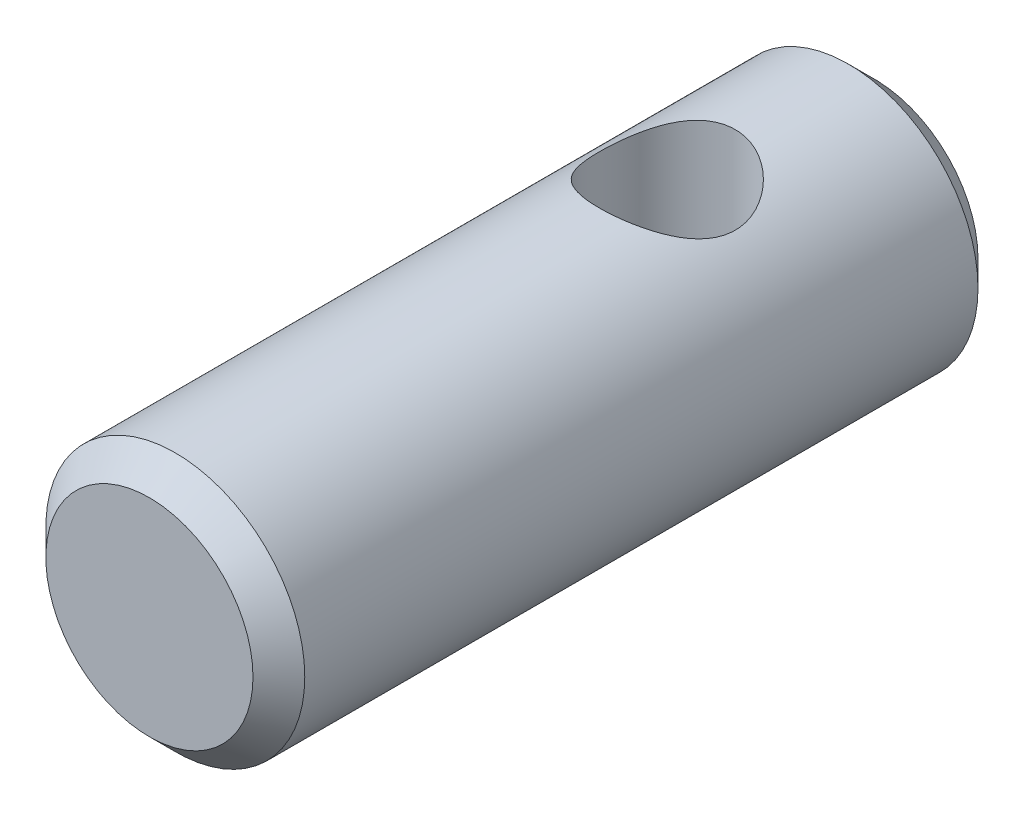
SolidWorks part; units mm, degrees
material "Plain Carbon Steel"
ref_plane "Front Plane" through (0, 0, 0) normal (0, 0, 1) x (1, 0, 0)
ref_plane "Top Plane" through (0, 0, 0) normal (0, 1, 0) x (1, 0, 0)
ref_plane "Right Plane" through (0, 0, 0) normal (1, 0, 0) x (0, 0, -1)
sketch "Pin Profile Ø20" plane through (0, 0, 0) normal (0, 0, 1) x (1, 0, 0)
  line L0 (0, 53.265) -> (0, -58.4616) construction
  line L1 (97.5044, 0) -> (-83.4189, 0) construction
  circle A0 centre (0, 0) radius 10
  dimension "D1" = 20
extrude "Pin Body Ø20x56" add sketch "Pin Profile Ø20" along normal blind 56
sketch "Cross Hole Sketch Ø10.5" plane through (0, 0, 0) normal (0, 1, 0) x (1, 0, 0)
  circle A0 centre (0, -16) radius 5.25
  dimension "D1" = 10.5
  dimension "D2" = 16
extrude "Cross Hole Ø10.5" cut sketch "Cross Hole Sketch Ø10.5" against normal mid plane 20
chamfer "End Chamfer 2x45°" distance 2 angle 45 2 edges at (10, 0, 56) (10, 0, 0)
